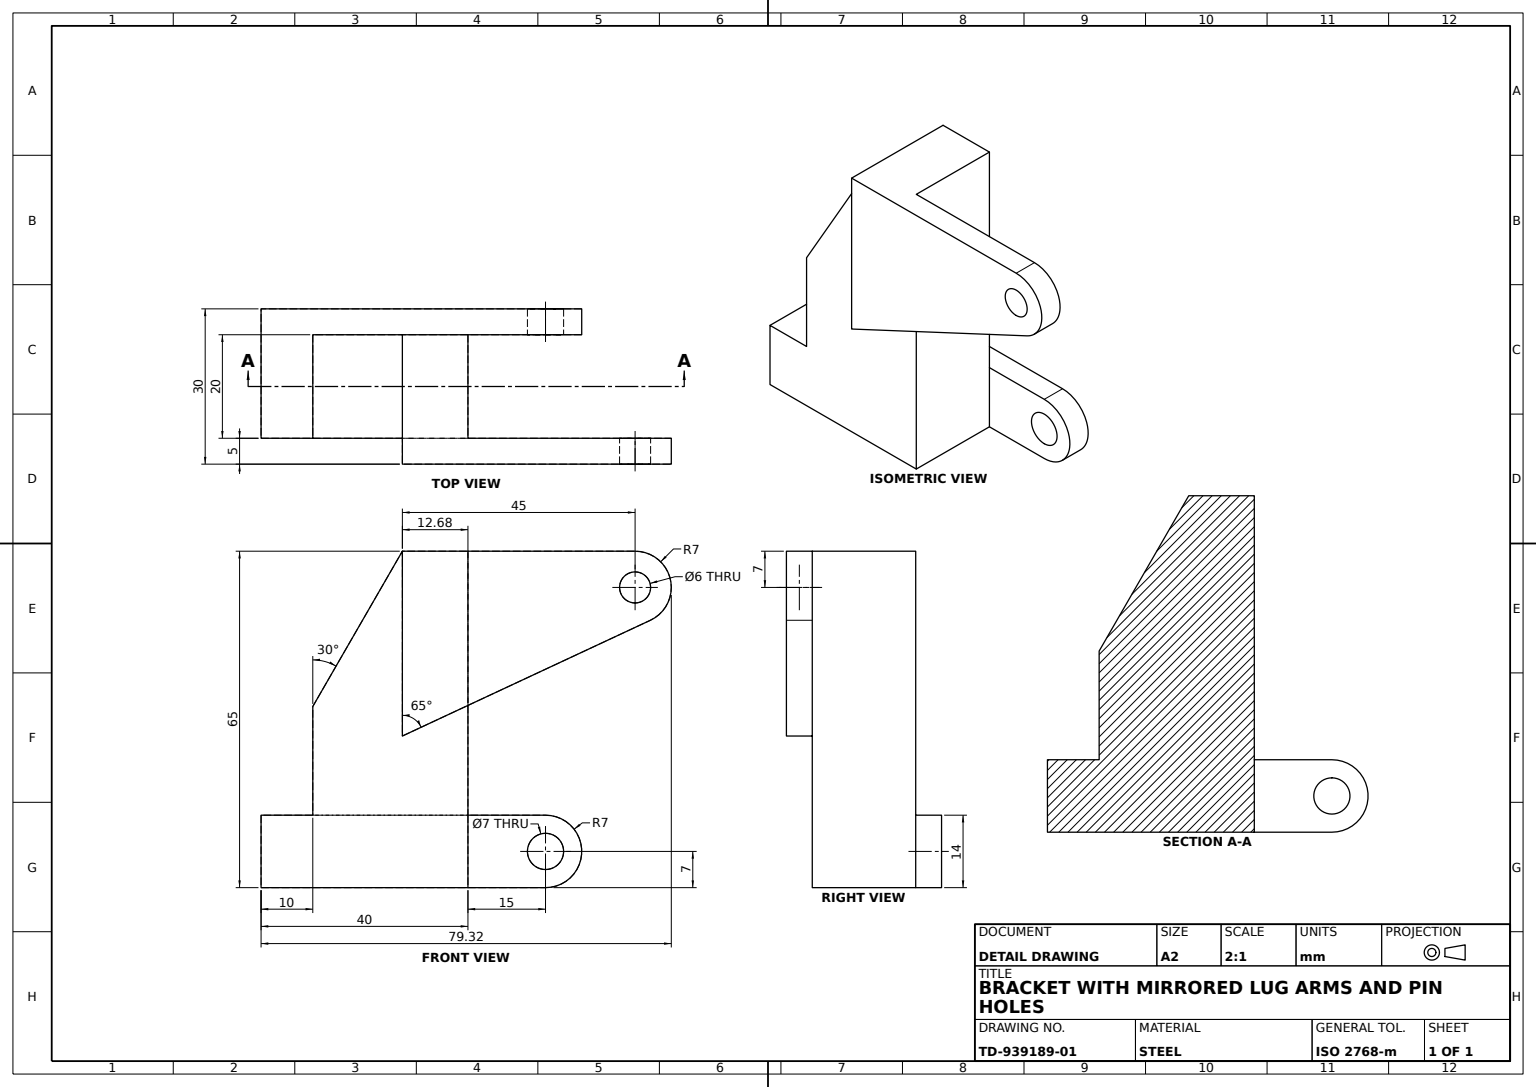
from build123d import *

# Parameters (mm, degrees)
BASE_BLOCK_SKETCH_W         = 20
BASE_BLOCK_SKETCH_H         = 65
BASE_BLOCK_DEPTH            = 40
ANGLED_CUT_30DEG_DEPTH      = 56.283360969
ANGLED_CUT_30DEG_DEPTH_BACK = 56.283360969
SIDE_PAD_DEPTH              = 5
PAD_TRIM_CUT_DEPTH          = 60.634302209
PAD_TRIM_CUT_DEPTH_BACK     = 5
PIN_HOLE_SKETCH_R           = 3.5
PIN_HOLE_7_DEPTH            = 5
LEVER_ARM_SKETCH_R          = 3
LEVER_ARM_DEPTH             = 5


with BuildPart() as part:
    # Base Block Sketch → Base Block (new body)
    with BuildSketch(Plane.XY):
        Rectangle(BASE_BLOCK_SKETCH_W, BASE_BLOCK_SKETCH_H)
    extrude(amount=BASE_BLOCK_DEPTH)

    # Angled Cut Sketch → Angled Cut 30deg (cut, two sides: drawn at the far end of the back side and taken through both)
    with BuildSketch(Plane(origin=(10, 0, 0), x_dir=(0, 0, -1), z_dir=(1, 0, 0)).offset(-ANGLED_CUT_30DEG_DEPTH_BACK)):
        Polygon((-12.679491924, 32.5), (-30, 2.5), (-30, -18.5), (-40, -18.5), (-40, 32.5), align=None)
    extrude(amount=ANGLED_CUT_30DEG_DEPTH + ANGLED_CUT_30DEG_DEPTH_BACK, mode=Mode.SUBTRACT)

    # Side Pad Sketch → Side Pad (add)
    with BuildSketch(Plane(origin=(10, 0, 0), x_dir=(0, 0, -1), z_dir=(1, 0, 0))):
        with BuildLine():
            Line((-40, -32.5), (15, -32.5))
            ThreePointArc((15, -32.5), (22, -25.5), (15, -18.5))
            Line((15, -18.5), (-40, -18.5))
            Line((-40, -18.5), (-40, -32.5))
        make_face()
    side_pad = extrude(amount=SIDE_PAD_DEPTH)

    # Side Pad Mirror: Side Pad across plane
    add(side_pad.mirror(Plane(origin=(0, 0, 0), x_dir=(0, 0, 1), z_dir=(1, 0, 0))))

    # Pad Trim Sketch → Pad Trim Cut (cut, two sides: drawn at the far end of the back side and taken through both)
    with BuildSketch(Plane(origin=(15, 0, 0), x_dir=(0, 0, -1), z_dir=(1, 0, 0)).offset(-PAD_TRIM_CUT_DEPTH_BACK)):
        with BuildLine():
            Line((-40, -18.5), (-40, -32.5))
            Line((-40, -32.5), (15, -32.5))
            ThreePointArc((15, -32.5), (22, -25.5), (15, -18.5))
            Line((15, -18.5), (-40, -18.5))
        make_face()
    extrude(amount=PAD_TRIM_CUT_DEPTH + PAD_TRIM_CUT_DEPTH_BACK, mode=Mode.SUBTRACT)

    # Pin Hole Sketch → Pin Hole Ø7 (cut)
    with BuildSketch(Plane(origin=(-10, 0, 0), x_dir=(0, 0, -1), z_dir=(1, 0, 0))):
        with Locations(Location((15, -25.5, 0), (0, 0, 90))):
            Circle(PIN_HOLE_SKETCH_R)
    extrude(amount=-PIN_HOLE_7_DEPTH, mode=Mode.SUBTRACT)

    # Lever Arm Sketch → Lever Arm (add)
    with BuildSketch(Plane(origin=(10, 0, 0), x_dir=(0, 0, -1), z_dir=(1, 0, 0))):
        with BuildLine():
            Line((-12.679491924, 32.5), (-12.679491924, -3.20749005))
            Line((-12.679491924, -3.20749005), (35.278835908, 19.155845491))
            ThreePointArc((35.278835908, 19.155845491), (39.154580126, 27.015077298), (32.320508076, 32.5))
            Line((32.320508076, 32.5), (-12.679491924, 32.5))
        make_face()
        with Locations(Location((32.320508076, 25.5, 0), (0, 0, 90))):
            Circle(LEVER_ARM_SKETCH_R, mode=Mode.SUBTRACT)
    extrude(amount=LEVER_ARM_DEPTH)


solid = part.part
